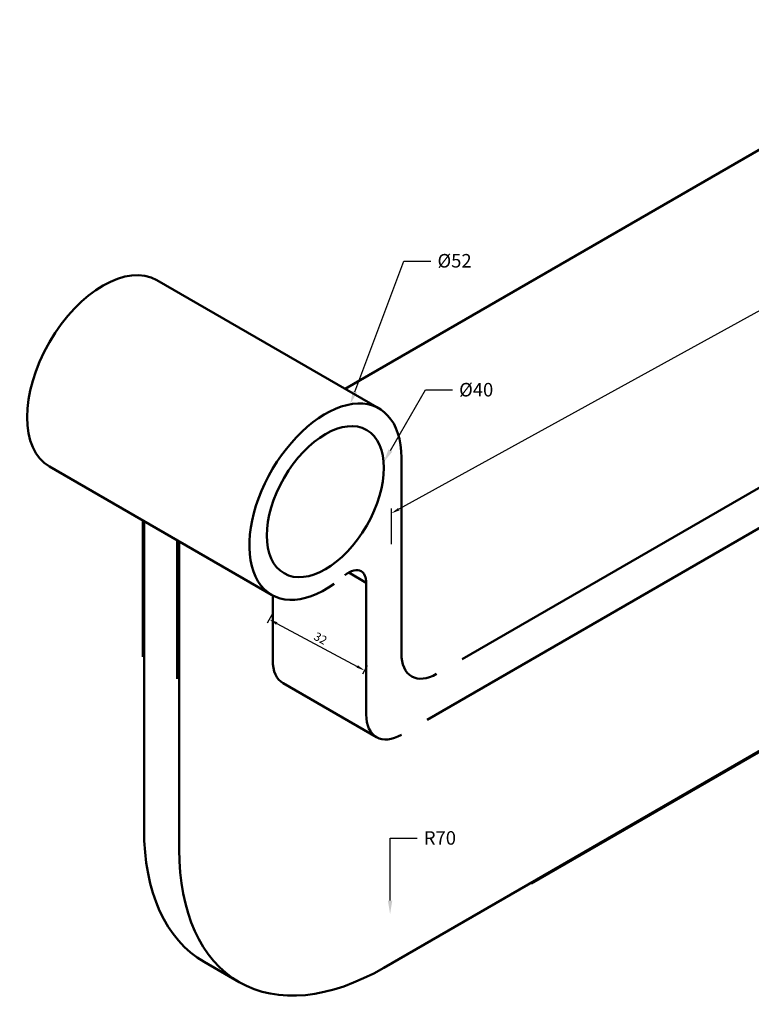
# Model space of a CAD drawing. Units: millimetres. Extents: x 3560 to 4017, y 1013 to 1432.
# Tile 1 of 2: x 3560 to 3777, y 1029 to 1320. Entities that reach past the tile are written whole.
import ezdxf
from ezdxf import colors
from ezdxf.entities.mleader import LeaderData, LeaderLine
from ezdxf.math import Vec2, Vec3

# ---------------------------------------------------------------- set-up
doc = ezdxf.new("R2010")
doc.units = ezdxf.units.MM
for name, color, linetype, lineweight in [('M-DIMS', 2, 'Continuous', 25), ('M-OUTL', 7, 'Continuous', 50), ('M-TEXT', 3, 'Continuous', 25)]:
    doc.layers.add(name, color=color, linetype=linetype, lineweight=lineweight)
doc.styles.get("Standard").update_dxf_attribs({"font": 'arial.ttf'})
doc.dimstyles.new('ISO-25', dxfattribs={"dimtxt": 2.5, "dimasz": 2.5, "dimexe": 1.25, "dimexo": 0.625, "dimtad": 1, "dimtxsty": 'Standard', "dimcen": 2.5, "dimadec": 0, "dimazin": 0, "dimtfac": 1, "dimtmove": 0, "dimatfit": 3, "dimfxl": 1, "dimarcsym": 0})

# ---------------------------------------------------------------- blocks, each defined once
blk = doc.blocks.new('*D11')
at = {"layer": 'Defpoints', "color": 0, "transparency": 16777216}
for p in [(3933.26, 1309.09), (3670.47, 1174.18), (3670.47, 1164.38)]:
    blk.add_point(p, dxfattribs=at)
at = {"layer": 'M-DIMS', "color": 0, "lineweight": -2, "transparency": 16777216}
for p, q in [((3931.07, 1317.69), (3672.66, 1175.38)), ((3933.26, 1309.8), (3933.26, 1320.32)), ((3670.47, 1165.09), (3670.47, 1175.61))]:
    blk.add_line(p, q, dxfattribs=at)
at = {"layer": 'M-DIMS', "color": 0, "transparency": 16777216}
for points in [[(3930.87, 1318.05), (3931.27, 1317.32), (3933.26, 1318.89)], [(3672.46, 1175.75), (3672.86, 1175.02), (3670.47, 1174.18)]]:
    blk.add_solid(points, dxfattribs=at)
at = {"layer": 'M-DIMS', "color": 0, "transparency": 16777216, "insert": (3800.95, 1248.2), "char_height": 2.5, "attachment_point": 5, "rotation": 28.8409}
blk.add_mtext('300', dxfattribs=at)
blk = doc.blocks.new('*D14')
at = {"layer": 'Defpoints', "color": 0, "transparency": 16777216}
for p in [(3635.34, 1144.64), (3663.57, 1129.55), (3662.55, 1127.66)]:
    blk.add_point(p, dxfattribs=at)
at = {"layer": 'M-DIMS', "color": 0, "lineweight": -2, "transparency": 16777216}
for p, q in [((3635.05, 1144.08), (3633.74, 1141.64)), ((3636.54, 1141.56), (3660.35, 1128.84)), ((3663.27, 1129), (3661.96, 1126.56))]:
    blk.add_line(p, q, dxfattribs=at)
at = {"layer": 'M-DIMS', "color": 0, "transparency": 16777216}
for points in [[(3636.73, 1141.93), (3636.34, 1141.2), (3634.33, 1142.74)], [(3660.55, 1129.2), (3660.15, 1128.47), (3662.55, 1127.66)]]:
    blk.add_solid(points, dxfattribs=at)
at = {"layer": 'M-DIMS', "color": 0, "transparency": 16777216, "insert": (3649.34, 1136.88), "char_height": 2.5, "attachment_point": 5, "rotation": 331.8751}
blk.add_mtext('32', dxfattribs=at)

msp = doc.modelspace()

# ---------------------------------------------------------------- linework, layer by layer
at = {"layer": 'M-OUTL'}
for p, q in [((3840.655, 1317.16), (3656.796, 1211.009)), ((3927.257, 1267.16), (3691.45, 1131.017)), ((3915.257, 1248.232), (3681.057, 1113.017)), ((3601.037, 1243.202), (3666.855, 1205.202)), ((3673.45, 1141.409), (3673.45, 1190.625)), ((3673.451, 1132.625), (3673.451, 1190.625)), ((3569.193, 1188.047), (3635.011, 1150.047)), ((3602.102, 1169.047), (3596.906, 1172.047)), ((3596.906, 1172.047), (3596.906, 1131.703)), ((3596.906, 1172.047), (3607.298, 1166.047)), ((3597.241, 1171.855), (3597.241, 1080.625)), ((3606.991, 1166.225), (3606.991, 1125.2)), ((3607.634, 1165.855), (3607.634, 1074.625)), ((3663.059, 1153.645), (3657.862, 1156.645)), ((3663.059, 1114.625), (3663.059, 1153.645)), ((3635.344, 1139.409), (3635.344, 1149.863)), ((3635.346, 1130.625), (3635.346, 1149.863)), ((3663.057, 1123.409), (3663.057, 1148.443)), ((3668.255, 1039.625), (3844.925, 1141.625)), ((3711.991, 1064.578), (3819.138, 1126.439)), ((3666.103, 1107.897), (3638.39, 1123.897)), ((3614.997, 1041.38), (3625.39, 1035.38))]:
    msp.add_line(p, q, dxfattribs=at)
for centre, major_axis, start_param, end_param in [((3585.115, 1215.625), (-15.922, -27.577), 3.1415927, 6.2831853), ((3650.933, 1177.625), (-15.922, -27.577), 2.3561945, 7.1860583), ((3657.864, 1150.647), (3.674, 6.363), 0, 1.0042143), ((3657.864, 1150.647), (3.674, 6.363), 5.497464, 6.2831853), ((3683.844, 1138.625), (-7.348, -12.728), 5.4977871, 6.2831853), ((3645.739, 1136.625), (7.348, 12.728), 2.3561945, 3.1415927), ((3683.844, 1138.625), (-7.348, -12.728), 0, 0.7853982), ((3673.451, 1120.625), (7.348, 12.728), 2.3561945, 3.1415927), ((3673.451, 1120.625), (7.348, 12.728), 3.1415927, 3.9269908), ((3657.864, 1115.627), (-42.867, -74.248), 5.4978103, 6.2831853), ((3668.257, 1109.627), (-42.867, -74.248), 5.4978103, 6.2831853), ((3668.257, 1109.627), (-42.867, -74.248), 0, 0.785375)]:
    msp.add_ellipse(centre, major_axis=major_axis, ratio=0.5773503, start_param=start_param, end_param=end_param, dxfattribs=at)
msp.add_ellipse((3650.933, 1177.625), major_axis=(-12.247, -21.213), ratio=0.5773503, dxfattribs=at)

# ---------------------------------------------------------------- dimensions: what is measured, and where the dimension line sits
at = {"layer": 'M-DIMS'}
for p1, p2, distance, picture, middle in [((3933.257, 1309.089), (3670.468, 1164.375), -8.588, '*D11', (3800.945, 1248.202)), ((3635.344, 1144.636), (3663.566, 1129.551), -2.148, '*D14', (3649.34, 1136.877))]:
    dim = msp.add_aligned_dim(p1=p1, p2=p2, distance=distance, dimstyle='ISO-25', override={"dimclrd": 0, "dimclre": 0, "dimclrt": 0}, dxfattribs=at)
    dim.commit()
    dim.dimension.update_dxf_attribs({"geometry": picture, "text_midpoint": middle})

# ---------------------------------------------------------------- leaders
at = {"layer": 'M-TEXT'}
ml = msp.add_multileader_mtext('Standard', dxfattribs=at)
ml.set_content('%%C52', color=256)
ml.set_leader_properties()
ml.build(insert=Vec2(0, 0))
ctx = ml.context
ctx.base_point, ctx.plane_origin = Vec3(3682.137, 1248.869), Vec3(3658.277, 1206.443)
notes = []
notes.append((ctx, [(0, (1, 1, 0), (3674.137, 1248.869), (1, 0), 8, [(0, [(3658.277, 1206.443)], 0, [])])]))
ctx.mtext.insert, ctx.mtext.flow_direction = Vec3(3684.137, 1250.95), 5
ml = msp.add_multileader_mtext('Standard', dxfattribs=at)
ml.set_content('%%C40', color=256)
ml.set_leader_properties()
ml.build(insert=Vec2(0, 0))
ctx = ml.context
ctx.base_point, ctx.plane_origin = Vec3(3688.547, 1210.697), Vec3(3668.19, 1189.294)
notes.append((ctx, [(0, (1, 1, 0), (3680.547, 1210.697), (1, 0), 8, [(0, [(3668.19, 1189.294)], 0, [])])]))
ctx.mtext.insert, ctx.mtext.flow_direction = Vec3(3690.547, 1212.778), 5
ml = msp.add_multileader_mtext('Standard', dxfattribs=at)
ml.set_content('R70', color=256)
ml.set_leader_properties()
ml.build(insert=Vec2(0, 0))
ctx = ml.context
ctx.base_point, ctx.plane_origin = Vec3(3678.098, 1078.04), Vec3(3670.098, 1055.54)
notes.append((ctx, [(0, (1, 1, 0), (3670.098, 1078.04), (1, 0), 8, [(0, [(3670.098, 1055.54)], 0, [])])]))
ctx.mtext.insert, ctx.mtext.flow_direction = Vec3(3680.098, 1080.074), 5
for ctx, leaders in notes:
    for number, flags, end, landing, length, lines in leaders:
        leader = LeaderData()
        leader.index, (leader.has_last_leader_line, leader.has_dogleg_vector, leader.attachment_direction) = number, flags
        leader.last_leader_point, leader.dogleg_vector, leader.dogleg_length = Vec3(end), Vec3(landing), length
        for number, points, colour, breaks in lines:
            line = LeaderLine()
            line.index, line.vertices, line.color, line.breaks = number, Vec3.list(points), colors.encode_raw_color(colour), breaks
            leader.lines.append(line)
        ctx.leaders.append(leader)

doc.saveas('drawing.dxf')
